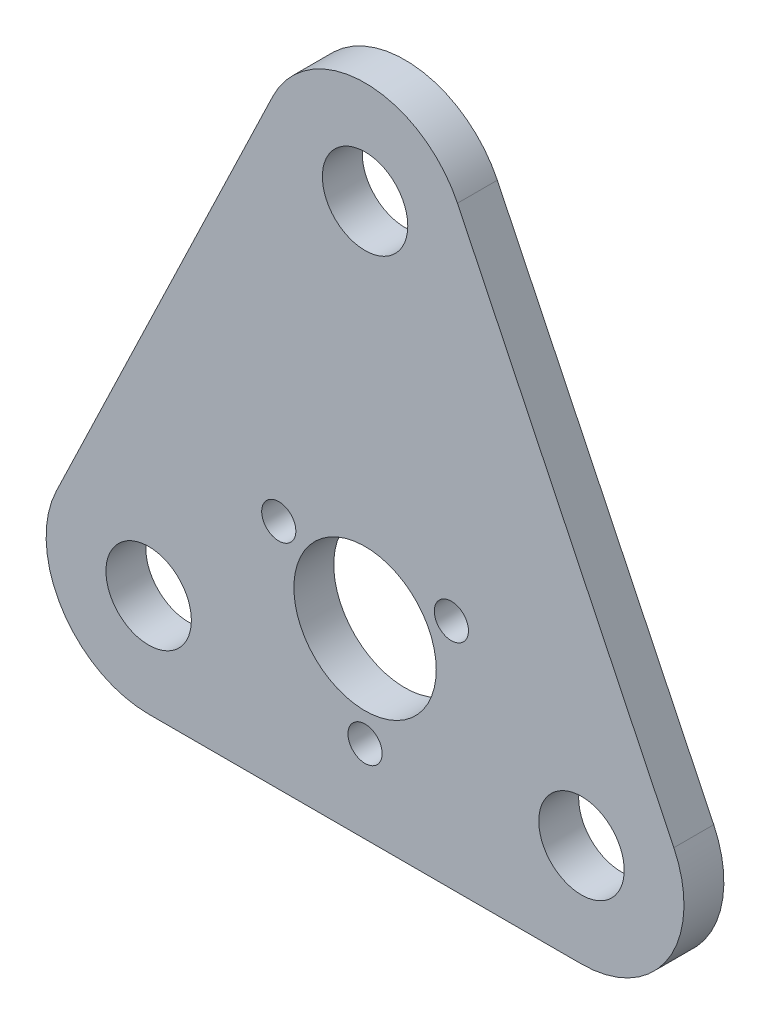
SolidWorks part; units mm, degrees
material "Plain Carbon Steel"
ref_plane "Front Plane" through (0, 0, 0) normal (0, 0, 1) x (1, 0, 0)
ref_plane "Top Plane" through (0, 0, 0) normal (0, 1, 0) x (1, 0, 0)
ref_plane "Right Plane" through (0, 0, 0) normal (1, 0, 0) x (0, 0, -1)
sketch "Plate Profile" plane through (0, 0, 0) normal (0, 0, 1) x (1, 0, 0)
  line L0 (-35.1686, 0) -> (24.765, 0) construction
  line L1 (0, 0) -> (0, 29.9008) construction
  line L2 (-38, -32) -> (38, -32)
  line L3 (-54.221, -6.1975) -> (-16.221, 72.8025)
  line L4 (54.221, -6.1975) -> (16.221, 72.8025)
  line L5 (0, 0) -> (-15.1554, 8.75) construction
  circle A0 centre (0, 0) radius 12.5
  circle A1 centre (0, 0) radius 17.5 construction
  circle A2 centre (0, -17.5) radius 3
  circle A3 centre (-15.1554, 8.75) radius 3
  circle A4 centre (15.1554, 8.75) radius 3
  circle A5 centre (-38, -14) radius 7.5
  arc A6 (-54.221, -6.1975) -> (-38, -32) centre (-38, -14) ccw
  circle A7 centre (38, -14) radius 7.5
  arc A8 (54.221, -6.1975) -> (38, -32) centre (38, -14) cw
  circle A9 centre (0, 65) radius 7.5
  arc A10 (16.221, 72.8025) -> (-16.221, 72.8025) centre (0, 65) ccw
  point P13 (0, 0)
  point P15 (0, 83)
  dimension "D1" = 25
  dimension "D2" = 35
  dimension "D3" = 6
  dimension "D5" = 15
  dimension "D7" = 36
  dimension "D9" = 15
  dimension "D10" = 36
  dimension "D6" = 38
  dimension "D8" = 32
  dimension "D11" = 115
  dimension "D4" = 3
extrude "Support Plate 7mm" add sketch "Plate Profile" along normal blind 7
